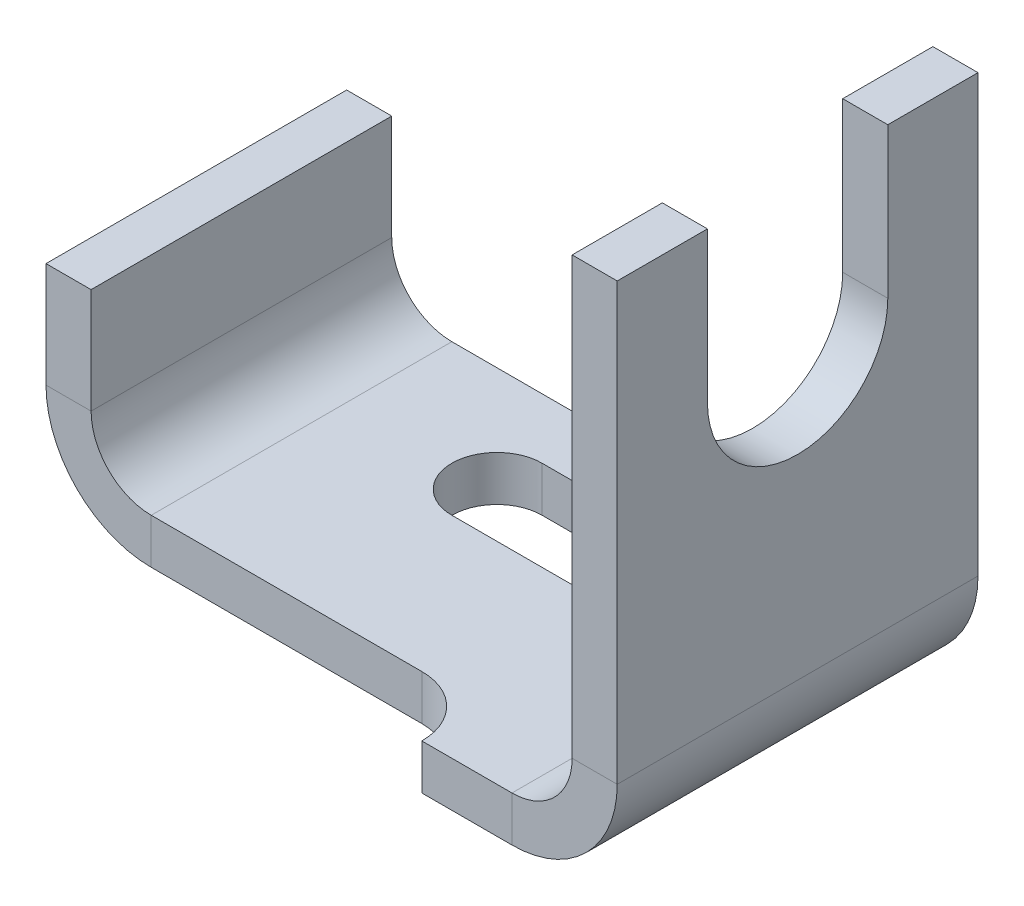
ISO-10303-21;
HEADER;
FILE_DESCRIPTION(('STEP AP214'),'2;1');
FILE_NAME('part.step','',(''),(''),'','','');
FILE_SCHEMA(('AUTOMOTIVE_DESIGN { 1 0 10303 214 1 1 1 1 }'));
ENDSEC;
DATA;
#1=APPLICATION_CONTEXT('core data for automotive mechanical design processes');
#2=APPLICATION_PROTOCOL_DEFINITION('international standard','automotive_design',2000,#1);
#3=PRODUCT_CONTEXT('',#1,'mechanical');
#4=PRODUCT('Part','Part','',(#3));
#5=PRODUCT_RELATED_PRODUCT_CATEGORY('part','',(#4));
#6=PRODUCT_DEFINITION_FORMATION('','',#4);
#7=PRODUCT_DEFINITION_CONTEXT('part definition',#1,'design');
#8=PRODUCT_DEFINITION('design','',#6,#7);
#9=PRODUCT_DEFINITION_SHAPE('','',#8);
#10=(LENGTH_UNIT() NAMED_UNIT(*) SI_UNIT(.MILLI.,.METRE.));
#11=(NAMED_UNIT(*) PLANE_ANGLE_UNIT() SI_UNIT($,.RADIAN.));
#12=(NAMED_UNIT(*) SI_UNIT($,.STERADIAN.) SOLID_ANGLE_UNIT());
#13=UNCERTAINTY_MEASURE_WITH_UNIT(LENGTH_MEASURE(1.E-05),#10,'distance_accuracy_value','');
#14=(GEOMETRIC_REPRESENTATION_CONTEXT(3) GLOBAL_UNCERTAINTY_ASSIGNED_CONTEXT((#13)) GLOBAL_UNIT_ASSIGNED_CONTEXT((#10,
#11,#12)) REPRESENTATION_CONTEXT('',''));
#15=CARTESIAN_POINT('',(0.,0.,0.));
#16=DIRECTION('',(0.,0.,1.));
#17=DIRECTION('',(1.,0.,0.));
#18=AXIS2_PLACEMENT_3D('',#15,#16,#17);
#19=CARTESIAN_POINT('',(18.,7.,12.));
#20=DIRECTION('',(0.,0.,1.));
#21=DIRECTION('',(1.,0.,0.));
#22=AXIS2_PLACEMENT_3D('',#19,#20,#21);
#23=PLANE('',#22);
#24=DIRECTION('',(1.,0.,0.));
#25=VECTOR('',#24,1.);
#26=CARTESIAN_POINT('',(0.,3.,12.));
#27=LINE('',#26,#25);
#28=CARTESIAN_POINT('',(14.,3.,12.));
#29=VERTEX_POINT('',#28);
#30=CARTESIAN_POINT('',(8.,3.,12.));
#31=VERTEX_POINT('',#30);
#32=EDGE_CURVE('E308',#29,#31,#27,.F.);
#33=ORIENTED_EDGE('',*,*,#32,.T.);
#34=DIRECTION('',(0.,1.,0.));
#35=VECTOR('',#34,1.);
#36=CARTESIAN_POINT('',(8.,3.,12.));
#37=LINE('',#36,#35);
#38=CARTESIAN_POINT('',(8.,0.,12.));
#39=VERTEX_POINT('',#38);
#40=EDGE_CURVE('E191',#31,#39,#37,.F.);
#41=ORIENTED_EDGE('',*,*,#40,.T.);
#42=DIRECTION('',(-1.,0.,0.));
#43=VECTOR('',#42,1.);
#44=CARTESIAN_POINT('',(0.,0.,12.));
#45=LINE('',#44,#43);
#46=CARTESIAN_POINT('',(14.,0.,12.));
#47=VERTEX_POINT('',#46);
#48=EDGE_CURVE('E287',#47,#39,#45,.T.);
#49=ORIENTED_EDGE('',*,*,#48,.F.);
#50=DIRECTION('',(0.,1.,0.));
#51=VECTOR('',#50,1.);
#52=CARTESIAN_POINT('',(14.,0.,12.));
#53=LINE('',#52,#51);
#54=EDGE_CURVE('E11',#47,#29,#53,.T.);
#55=ORIENTED_EDGE('',*,*,#54,.T.);
#56=EDGE_LOOP('',(#33,#41,#49,#55));
#57=FACE_BOUND('',#56,.T.);
#58=ADVANCED_FACE('F41',(#57),#23,.T.);
#59=CARTESIAN_POINT('',(-18.,0.,12.));
#60=DIRECTION('',(-1.,0.,0.));
#61=DIRECTION('',(0.,0.,1.));
#62=AXIS2_PLACEMENT_3D('',#59,#60,#61);
#63=PLANE('',#62);
#64=DIRECTION('',(0.,1.,0.));
#65=VECTOR('',#64,1.);
#66=CARTESIAN_POINT('',(-18.,0.,8.));
#67=LINE('',#66,#65);
#68=CARTESIAN_POINT('',(-18.,7.,8.));
#69=VERTEX_POINT('',#68);
#70=CARTESIAN_POINT('',(-18.,14.,8.));
#71=VERTEX_POINT('',#70);
#72=EDGE_CURVE('E227',#69,#71,#67,.T.);
#73=ORIENTED_EDGE('',*,*,#72,.F.);
#74=DIRECTION('',(0.,0.,-1.));
#75=VECTOR('',#74,1.);
#76=CARTESIAN_POINT('',(-18.,7.,12.));
#77=LINE('',#76,#75);
#78=CARTESIAN_POINT('',(-18.,7.,-12.));
#79=VERTEX_POINT('',#78);
#80=EDGE_CURVE('E309',#69,#79,#77,.T.);
#81=ORIENTED_EDGE('',*,*,#80,.T.);
#82=DIRECTION('',(0.,1.,0.));
#83=VECTOR('',#82,1.);
#84=CARTESIAN_POINT('',(-18.,0.,-12.));
#85=LINE('',#84,#83);
#86=CARTESIAN_POINT('',(-18.,14.,-12.));
#87=VERTEX_POINT('',#86);
#88=EDGE_CURVE('E282',#79,#87,#85,.T.);
#89=ORIENTED_EDGE('',*,*,#88,.T.);
#90=DIRECTION('',(0.,0.,-1.));
#91=VECTOR('',#90,1.);
#92=CARTESIAN_POINT('',(-18.,14.,12.));
#93=LINE('',#92,#91);
#94=EDGE_CURVE('E375',#71,#87,#93,.T.);
#95=ORIENTED_EDGE('',*,*,#94,.F.);
#96=EDGE_LOOP('',(#73,#81,#89,#95));
#97=FACE_BOUND('',#96,.T.);
#98=ADVANCED_FACE('F455',(#97),#63,.F.);
#99=CARTESIAN_POINT('',(-21.,14.,12.));
#100=DIRECTION('',(0.,1.,0.));
#101=DIRECTION('',(0.,0.,1.));
#102=AXIS2_PLACEMENT_3D('',#99,#100,#101);
#103=PLANE('',#102);
#104=DIRECTION('',(0.,0.,-1.));
#105=VECTOR('',#104,1.);
#106=CARTESIAN_POINT('',(-21.,14.,12.));
#107=LINE('',#106,#105);
#108=CARTESIAN_POINT('',(-21.,14.,8.));
#109=VERTEX_POINT('',#108);
#110=CARTESIAN_POINT('',(-21.,14.,-12.));
#111=VERTEX_POINT('',#110);
#112=EDGE_CURVE('E369',#109,#111,#107,.T.);
#113=ORIENTED_EDGE('',*,*,#112,.F.);
#114=DIRECTION('',(-1.,0.,0.));
#115=VECTOR('',#114,1.);
#116=CARTESIAN_POINT('',(-21.,14.,8.));
#117=LINE('',#116,#115);
#118=EDGE_CURVE('E230',#109,#71,#117,.F.);
#119=ORIENTED_EDGE('',*,*,#118,.T.);
#120=ORIENTED_EDGE('',*,*,#94,.T.);
#121=DIRECTION('',(1.,0.,0.));
#122=VECTOR('',#121,1.);
#123=CARTESIAN_POINT('',(-21.,14.,-12.));
#124=LINE('',#123,#122);
#125=EDGE_CURVE('E312',#111,#87,#124,.T.);
#126=ORIENTED_EDGE('',*,*,#125,.F.);
#127=EDGE_LOOP('',(#113,#119,#120,#126));
#128=FACE_BOUND('',#127,.T.);
#129=ADVANCED_FACE('F456',(#128),#103,.T.);
#130=CARTESIAN_POINT('',(-21.,0.,12.));
#131=DIRECTION('',(-1.,0.,0.));
#132=DIRECTION('',(0.,0.,1.));
#133=AXIS2_PLACEMENT_3D('',#130,#131,#132);
#134=PLANE('',#133);
#135=DIRECTION('',(0.,0.,-1.));
#136=VECTOR('',#135,1.);
#137=CARTESIAN_POINT('',(-21.,7.,12.));
#138=LINE('',#137,#136);
#139=CARTESIAN_POINT('',(-21.,7.00000000000001,8.));
#140=VERTEX_POINT('',#139);
#141=CARTESIAN_POINT('',(-21.,7.,-12.));
#142=VERTEX_POINT('',#141);
#143=EDGE_CURVE('E368',#140,#142,#138,.T.);
#144=ORIENTED_EDGE('',*,*,#143,.F.);
#145=DIRECTION('',(0.,1.,0.));
#146=VECTOR('',#145,1.);
#147=CARTESIAN_POINT('',(-21.,0.,8.));
#148=LINE('',#147,#146);
#149=EDGE_CURVE('E222',#140,#109,#148,.T.);
#150=ORIENTED_EDGE('',*,*,#149,.T.);
#151=ORIENTED_EDGE('',*,*,#112,.T.);
#152=DIRECTION('',(0.,1.,0.));
#153=VECTOR('',#152,1.);
#154=CARTESIAN_POINT('',(-21.,0.,-12.));
#155=LINE('',#154,#153);
#156=EDGE_CURVE('E317',#142,#111,#155,.T.);
#157=ORIENTED_EDGE('',*,*,#156,.F.);
#158=EDGE_LOOP('',(#144,#150,#151,#157));
#159=FACE_BOUND('',#158,.T.);
#160=ADVANCED_FACE('F476',(#159),#134,.T.);
#161=CARTESIAN_POINT('',(-14.,7.,12.));
#162=DIRECTION('',(0.,0.,-1.));
#163=DIRECTION('',(-1.,0.,0.));
#164=AXIS2_PLACEMENT_3D('',#161,#162,#163);
#165=CYLINDRICAL_SURFACE('',#164,7.);
#166=DIRECTION('',(0.,0.,-1.));
#167=VECTOR('',#166,1.);
#168=CARTESIAN_POINT('',(-14.,0.,12.));
#169=LINE('',#168,#167);
#170=CARTESIAN_POINT('',(-14.,0.,8.));
#171=VERTEX_POINT('',#170);
#172=CARTESIAN_POINT('',(-14.,0.,-12.));
#173=VERTEX_POINT('',#172);
#174=EDGE_CURVE('E366',#171,#173,#169,.T.);
#175=ORIENTED_EDGE('',*,*,#174,.F.);
#176=CARTESIAN_POINT('',(-14.,7.,8.));
#177=DIRECTION('',(0.,0.,-1.));
#178=DIRECTION('',(-1.,0.,0.));
#179=AXIS2_PLACEMENT_3D('',#176,#177,#178);
#180=CIRCLE('',#179,7.);
#181=EDGE_CURVE('E223',#171,#140,#180,.T.);
#182=ORIENTED_EDGE('',*,*,#181,.T.);
#183=ORIENTED_EDGE('',*,*,#143,.T.);
#184=CARTESIAN_POINT('',(-14.,7.,-12.));
#185=DIRECTION('',(0.,0.,1.));
#186=DIRECTION('',(1.,0.,0.));
#187=AXIS2_PLACEMENT_3D('',#184,#185,#186);
#188=CIRCLE('',#187,7.);
#189=EDGE_CURVE('E316',#173,#142,#188,.F.);
#190=ORIENTED_EDGE('',*,*,#189,.F.);
#191=EDGE_LOOP('',(#175,#182,#183,#190));
#192=FACE_BOUND('',#191,.T.);
#193=ADVANCED_FACE('F480',(#192),#165,.T.);
#194=CARTESIAN_POINT('',(0.,0.,12.));
#195=DIRECTION('',(0.,-1.,0.));
#196=DIRECTION('',(0.,0.,-1.));
#197=AXIS2_PLACEMENT_3D('',#194,#195,#196);
#198=PLANE('',#197);
#199=CARTESIAN_POINT('',(-3.99999999999999,0.,-5.));
#200=DIRECTION('',(0.,1.,0.));
#201=DIRECTION('',(-1.,0.,0.));
#202=AXIS2_PLACEMENT_3D('',#199,#200,#201);
#203=CIRCLE('',#202,3.);
#204=CARTESIAN_POINT('',(-3.99999999999999,0.,-8.));
#205=VERTEX_POINT('',#204);
#206=CARTESIAN_POINT('',(-3.99999999999999,0.,-2.));
#207=VERTEX_POINT('',#206);
#208=EDGE_CURVE('E231',#205,#207,#203,.T.);
#209=ORIENTED_EDGE('',*,*,#208,.T.);
#210=DIRECTION('',(1.,0.,0.));
#211=VECTOR('',#210,1.);
#212=CARTESIAN_POINT('',(-3.99999999999999,0.,-2.));
#213=LINE('',#212,#211);
#214=CARTESIAN_POINT('',(8.00000000000001,0.,-2.));
#215=VERTEX_POINT('',#214);
#216=EDGE_CURVE('E236',#207,#215,#213,.T.);
#217=ORIENTED_EDGE('',*,*,#216,.T.);
#218=CARTESIAN_POINT('',(8.00000000000001,0.,-5.));
#219=DIRECTION('',(0.,1.,0.));
#220=DIRECTION('',(-1.,0.,0.));
#221=AXIS2_PLACEMENT_3D('',#218,#219,#220);
#222=CIRCLE('',#221,3.);
#223=CARTESIAN_POINT('',(8.00000000000001,0.,-8.));
#224=VERTEX_POINT('',#223);
#225=EDGE_CURVE('E65',#215,#224,#222,.T.);
#226=ORIENTED_EDGE('',*,*,#225,.T.);
#227=DIRECTION('',(-1.,0.,0.));
#228=VECTOR('',#227,1.);
#229=CARTESIAN_POINT('',(-3.99999999999999,0.,-8.));
#230=LINE('',#229,#228);
#231=EDGE_CURVE('E241',#224,#205,#230,.T.);
#232=ORIENTED_EDGE('',*,*,#231,.T.);
#233=EDGE_LOOP('',(#209,#217,#226,#232));
#234=FACE_BOUND('',#233,.T.);
#235=ORIENTED_EDGE('',*,*,#48,.T.);
#236=CARTESIAN_POINT('',(4.,0.,12.));
#237=DIRECTION('',(0.,-1.,0.));
#238=DIRECTION('',(1.,0.,0.));
#239=AXIS2_PLACEMENT_3D('',#236,#237,#238);
#240=CIRCLE('',#239,4.);
#241=CARTESIAN_POINT('',(4.,0.,8.));
#242=VERTEX_POINT('',#241);
#243=EDGE_CURVE('E202',#242,#39,#240,.T.);
#244=ORIENTED_EDGE('',*,*,#243,.F.);
#245=DIRECTION('',(1.,0.,0.));
#246=VECTOR('',#245,1.);
#247=CARTESIAN_POINT('',(0.,0.,8.));
#248=LINE('',#247,#246);
#249=EDGE_CURVE('E204',#171,#242,#248,.T.);
#250=ORIENTED_EDGE('',*,*,#249,.F.);
#251=ORIENTED_EDGE('',*,*,#174,.T.);
#252=DIRECTION('',(-1.,0.,0.));
#253=VECTOR('',#252,1.);
#254=CARTESIAN_POINT('',(0.,0.,-12.));
#255=LINE('',#254,#253);
#256=CARTESIAN_POINT('',(14.,0.,-12.));
#257=VERTEX_POINT('',#256);
#258=EDGE_CURVE('E324',#257,#173,#255,.T.);
#259=ORIENTED_EDGE('',*,*,#258,.F.);
#260=DIRECTION('',(0.,0.,-1.));
#261=VECTOR('',#260,1.);
#262=CARTESIAN_POINT('',(14.,0.,12.));
#263=LINE('',#262,#261);
#264=EDGE_CURVE('E361',#47,#257,#263,.T.);
#265=ORIENTED_EDGE('',*,*,#264,.F.);
#266=EDGE_LOOP('',(#235,#244,#250,#251,#259,#265));
#267=FACE_BOUND('',#266,.T.);
#268=ADVANCED_FACE('F415',(#234,#267),#198,.T.);
#269=CARTESIAN_POINT('',(0.,3.,12.));
#270=DIRECTION('',(0.,-1.,0.));
#271=DIRECTION('',(1.,0.,0.));
#272=AXIS2_PLACEMENT_3D('',#269,#270,#271);
#273=PLANE('',#272);
#274=DIRECTION('',(1.,0.,0.));
#275=VECTOR('',#274,1.);
#276=CARTESIAN_POINT('',(-3.99999999999999,3.,-2.));
#277=LINE('',#276,#275);
#278=CARTESIAN_POINT('',(-3.99999999999999,3.,-2.));
#279=VERTEX_POINT('',#278);
#280=CARTESIAN_POINT('',(8.00000000000001,3.,-2.));
#281=VERTEX_POINT('',#280);
#282=EDGE_CURVE('E246',#279,#281,#277,.T.);
#283=ORIENTED_EDGE('',*,*,#282,.F.);
#284=CARTESIAN_POINT('',(-3.99999999999999,3.,-5.));
#285=DIRECTION('',(0.,1.,0.));
#286=DIRECTION('',(-1.,0.,0.));
#287=AXIS2_PLACEMENT_3D('',#284,#285,#286);
#288=CIRCLE('',#287,3.);
#289=CARTESIAN_POINT('',(-3.99999999999999,3.,-8.));
#290=VERTEX_POINT('',#289);
#291=EDGE_CURVE('E235',#290,#279,#288,.T.);
#292=ORIENTED_EDGE('',*,*,#291,.F.);
#293=DIRECTION('',(-1.,0.,0.));
#294=VECTOR('',#293,1.);
#295=CARTESIAN_POINT('',(-3.99999999999999,3.,-8.));
#296=LINE('',#295,#294);
#297=CARTESIAN_POINT('',(8.00000000000001,3.,-8.));
#298=VERTEX_POINT('',#297);
#299=EDGE_CURVE('E240',#298,#290,#296,.T.);
#300=ORIENTED_EDGE('',*,*,#299,.F.);
#301=CARTESIAN_POINT('',(8.00000000000001,3.,-5.));
#302=DIRECTION('',(0.,1.,0.));
#303=DIRECTION('',(-1.,0.,0.));
#304=AXIS2_PLACEMENT_3D('',#301,#302,#303);
#305=CIRCLE('',#304,3.);
#306=EDGE_CURVE('E248',#281,#298,#305,.T.);
#307=ORIENTED_EDGE('',*,*,#306,.F.);
#308=EDGE_LOOP('',(#283,#292,#300,#307));
#309=FACE_BOUND('',#308,.T.);
#310=CARTESIAN_POINT('',(4.,3.,12.));
#311=DIRECTION('',(0.,-1.,0.));
#312=DIRECTION('',(1.,0.,0.));
#313=AXIS2_PLACEMENT_3D('',#310,#311,#312);
#314=CIRCLE('',#313,4.);
#315=CARTESIAN_POINT('',(4.,3.,8.));
#316=VERTEX_POINT('',#315);
#317=EDGE_CURVE('E188',#316,#31,#314,.T.);
#318=ORIENTED_EDGE('',*,*,#317,.T.);
#319=ORIENTED_EDGE('',*,*,#32,.F.);
#320=DIRECTION('',(0.,0.,-1.));
#321=VECTOR('',#320,1.);
#322=CARTESIAN_POINT('',(14.,3.,12.));
#323=LINE('',#322,#321);
#324=CARTESIAN_POINT('',(14.,3.,-12.));
#325=VERTEX_POINT('',#324);
#326=EDGE_CURVE('E346',#29,#325,#323,.T.);
#327=ORIENTED_EDGE('',*,*,#326,.T.);
#328=DIRECTION('',(-1.,0.,0.));
#329=VECTOR('',#328,1.);
#330=CARTESIAN_POINT('',(0.,3.,-12.));
#331=LINE('',#330,#329);
#332=CARTESIAN_POINT('',(-14.,3.,-12.));
#333=VERTEX_POINT('',#332);
#334=EDGE_CURVE('E338',#325,#333,#331,.T.);
#335=ORIENTED_EDGE('',*,*,#334,.T.);
#336=DIRECTION('',(0.,0.,-1.));
#337=VECTOR('',#336,1.);
#338=CARTESIAN_POINT('',(-14.,3.,12.));
#339=LINE('',#338,#337);
#340=CARTESIAN_POINT('',(-14.,3.,8.));
#341=VERTEX_POINT('',#340);
#342=EDGE_CURVE('E206',#341,#333,#339,.T.);
#343=ORIENTED_EDGE('',*,*,#342,.F.);
#344=DIRECTION('',(1.,0.,0.));
#345=VECTOR('',#344,1.);
#346=CARTESIAN_POINT('',(0.,3.,8.));
#347=LINE('',#346,#345);
#348=EDGE_CURVE('E57',#341,#316,#347,.T.);
#349=ORIENTED_EDGE('',*,*,#348,.T.);
#350=EDGE_LOOP('',(#318,#319,#327,#335,#343,#349));
#351=FACE_BOUND('',#350,.T.);
#352=ADVANCED_FACE('F207',(#309,#351),#273,.F.);
#353=CARTESIAN_POINT('',(-14.,7.,12.));
#354=DIRECTION('',(0.,0.,-1.));
#355=DIRECTION('',(-1.,0.,0.));
#356=AXIS2_PLACEMENT_3D('',#353,#354,#355);
#357=CYLINDRICAL_SURFACE('',#356,4.);
#358=CARTESIAN_POINT('',(-14.,7.,8.));
#359=DIRECTION('',(0.,0.,-1.));
#360=DIRECTION('',(-1.,0.,0.));
#361=AXIS2_PLACEMENT_3D('',#358,#359,#360);
#362=CIRCLE('',#361,4.);
#363=EDGE_CURVE('E216',#341,#69,#362,.T.);
#364=ORIENTED_EDGE('',*,*,#363,.F.);
#365=ORIENTED_EDGE('',*,*,#342,.T.);
#366=CARTESIAN_POINT('',(-14.,7.,-12.));
#367=DIRECTION('',(0.,0.,1.));
#368=DIRECTION('',(1.,0.,0.));
#369=AXIS2_PLACEMENT_3D('',#366,#367,#368);
#370=CIRCLE('',#369,4.);
#371=EDGE_CURVE('E291',#333,#79,#370,.F.);
#372=ORIENTED_EDGE('',*,*,#371,.T.);
#373=ORIENTED_EDGE('',*,*,#80,.F.);
#374=EDGE_LOOP('',(#364,#365,#372,#373));
#375=FACE_BOUND('',#374,.T.);
#376=ADVANCED_FACE('F497',(#375),#357,.F.);
#377=CARTESIAN_POINT('',(18.,36.,12.));
#378=DIRECTION('',(0.,1.,0.));
#379=DIRECTION('',(0.,0.,1.));
#380=AXIS2_PLACEMENT_3D('',#377,#378,#379);
#381=PLANE('',#380);
#382=DIRECTION('',(-1.,0.,0.));
#383=VECTOR('',#382,1.);
#384=CARTESIAN_POINT('',(21.,36.,6.));
#385=LINE('',#384,#383);
#386=CARTESIAN_POINT('',(21.,36.,6.));
#387=VERTEX_POINT('',#386);
#388=CARTESIAN_POINT('',(18.,36.,6.));
#389=VERTEX_POINT('',#388);
#390=EDGE_CURVE('E271',#387,#389,#385,.T.);
#391=ORIENTED_EDGE('',*,*,#390,.T.);
#392=DIRECTION('',(0.,0.,-1.));
#393=VECTOR('',#392,1.);
#394=CARTESIAN_POINT('',(18.,36.,12.));
#395=LINE('',#394,#393);
#396=CARTESIAN_POINT('',(18.,36.,12.));
#397=VERTEX_POINT('',#396);
#398=EDGE_CURVE('E351',#397,#389,#395,.T.);
#399=ORIENTED_EDGE('',*,*,#398,.F.);
#400=DIRECTION('',(1.,0.,0.));
#401=VECTOR('',#400,1.);
#402=CARTESIAN_POINT('',(18.,36.,12.));
#403=LINE('',#402,#401);
#404=CARTESIAN_POINT('',(21.,36.,12.));
#405=VERTEX_POINT('',#404);
#406=EDGE_CURVE('E299',#397,#405,#403,.T.);
#407=ORIENTED_EDGE('',*,*,#406,.T.);
#408=DIRECTION('',(0.,0.,-1.));
#409=VECTOR('',#408,1.);
#410=CARTESIAN_POINT('',(21.,36.,12.));
#411=LINE('',#410,#409);
#412=EDGE_CURVE('E357',#405,#387,#411,.T.);
#413=ORIENTED_EDGE('',*,*,#412,.T.);
#414=EDGE_LOOP('',(#391,#399,#407,#413));
#415=FACE_BOUND('',#414,.T.);
#416=ADVANCED_FACE('F402',(#415),#381,.T.);
#417=CARTESIAN_POINT('',(14.,0.,12.));
#418=DIRECTION('',(0.,0.,1.));
#419=DIRECTION('',(1.,0.,0.));
#420=AXIS2_PLACEMENT_3D('',#417,#418,#419);
#421=PLANE('',#420);
#422=ORIENTED_EDGE('',*,*,#54,.F.);
#423=CARTESIAN_POINT('',(14.,7.,12.));
#424=DIRECTION('',(0.,0.,1.));
#425=DIRECTION('',(1.,0.,0.));
#426=AXIS2_PLACEMENT_3D('',#423,#424,#425);
#427=CIRCLE('',#426,7.);
#428=CARTESIAN_POINT('',(21.,7.,12.));
#429=VERTEX_POINT('',#428);
#430=EDGE_CURVE('E292',#429,#47,#427,.F.);
#431=ORIENTED_EDGE('',*,*,#430,.F.);
#432=DIRECTION('',(1.,0.,0.));
#433=VECTOR('',#432,1.);
#434=CARTESIAN_POINT('',(18.,7.,12.));
#435=LINE('',#434,#433);
#436=CARTESIAN_POINT('',(18.,7.,12.));
#437=VERTEX_POINT('',#436);
#438=EDGE_CURVE('E47',#437,#429,#435,.T.);
#439=ORIENTED_EDGE('',*,*,#438,.F.);
#440=CARTESIAN_POINT('',(14.,7.,12.));
#441=DIRECTION('',(0.,0.,1.));
#442=DIRECTION('',(1.,0.,0.));
#443=AXIS2_PLACEMENT_3D('',#440,#441,#442);
#444=CIRCLE('',#443,4.);
#445=EDGE_CURVE('E304',#437,#29,#444,.F.);
#446=ORIENTED_EDGE('',*,*,#445,.T.);
#447=EDGE_LOOP('',(#422,#431,#439,#446));
#448=FACE_BOUND('',#447,.T.);
#449=ADVANCED_FACE('F43',(#448),#421,.T.);
#450=CARTESIAN_POINT('',(21.,7.,-12.));
#451=DIRECTION('',(0.,0.,-1.));
#452=DIRECTION('',(-1.,0.,0.));
#453=AXIS2_PLACEMENT_3D('',#450,#451,#452);
#454=PLANE('',#453);
#455=DIRECTION('',(-1.,0.,0.));
#456=VECTOR('',#455,1.);
#457=CARTESIAN_POINT('',(21.,7.,-12.));
#458=LINE('',#457,#456);
#459=CARTESIAN_POINT('',(21.,7.,-12.));
#460=VERTEX_POINT('',#459);
#461=CARTESIAN_POINT('',(18.,7.,-12.));
#462=VERTEX_POINT('',#461);
#463=EDGE_CURVE('E385',#460,#462,#458,.T.);
#464=ORIENTED_EDGE('',*,*,#463,.F.);
#465=CARTESIAN_POINT('',(14.,7.,-12.));
#466=DIRECTION('',(0.,0.,1.));
#467=DIRECTION('',(1.,0.,0.));
#468=AXIS2_PLACEMENT_3D('',#465,#466,#467);
#469=CIRCLE('',#468,7.);
#470=EDGE_CURVE('E321',#460,#257,#469,.F.);
#471=ORIENTED_EDGE('',*,*,#470,.T.);
#472=DIRECTION('',(0.,-1.,0.));
#473=VECTOR('',#472,1.);
#474=CARTESIAN_POINT('',(14.,3.,-12.));
#475=LINE('',#474,#473);
#476=EDGE_CURVE('E379',#325,#257,#475,.T.);
#477=ORIENTED_EDGE('',*,*,#476,.F.);
#478=CARTESIAN_POINT('',(14.,7.,-12.));
#479=DIRECTION('',(0.,0.,1.));
#480=DIRECTION('',(1.,0.,0.));
#481=AXIS2_PLACEMENT_3D('',#478,#479,#480);
#482=CIRCLE('',#481,4.);
#483=EDGE_CURVE('E340',#462,#325,#482,.F.);
#484=ORIENTED_EDGE('',*,*,#483,.F.);
#485=EDGE_LOOP('',(#464,#471,#477,#484));
#486=FACE_BOUND('',#485,.T.);
#487=ADVANCED_FACE('F423',(#486),#454,.T.);
#488=CARTESIAN_POINT('',(14.,3.,-12.));
#489=DIRECTION('',(0.,0.,-1.));
#490=DIRECTION('',(-1.,0.,0.));
#491=AXIS2_PLACEMENT_3D('',#488,#489,#490);
#492=PLANE('',#491);
#493=DIRECTION('',(0.,-1.,0.));
#494=VECTOR('',#493,1.);
#495=CARTESIAN_POINT('',(21.,0.,-12.));
#496=LINE('',#495,#494);
#497=CARTESIAN_POINT('',(21.,36.,-12.));
#498=VERTEX_POINT('',#497);
#499=EDGE_CURVE('E330',#498,#460,#496,.T.);
#500=ORIENTED_EDGE('',*,*,#499,.T.);
#501=ORIENTED_EDGE('',*,*,#463,.T.);
#502=DIRECTION('',(0.,1.,0.));
#503=VECTOR('',#502,1.);
#504=CARTESIAN_POINT('',(18.,0.,-12.));
#505=LINE('',#504,#503);
#506=CARTESIAN_POINT('',(18.,36.,-12.));
#507=VERTEX_POINT('',#506);
#508=EDGE_CURVE('E335',#507,#462,#505,.F.);
#509=ORIENTED_EDGE('',*,*,#508,.F.);
#510=DIRECTION('',(1.,0.,0.));
#511=VECTOR('',#510,1.);
#512=CARTESIAN_POINT('',(18.,36.,-12.));
#513=LINE('',#512,#511);
#514=EDGE_CURVE('E333',#507,#498,#513,.T.);
#515=ORIENTED_EDGE('',*,*,#514,.T.);
#516=EDGE_LOOP('',(#500,#501,#509,#515));
#517=FACE_BOUND('',#516,.T.);
#518=ADVANCED_FACE('F425',(#517),#492,.T.);
#519=CARTESIAN_POINT('',(-14.,0.,-12.));
#520=DIRECTION('',(0.,0.,-1.));
#521=DIRECTION('',(-1.,0.,0.));
#522=AXIS2_PLACEMENT_3D('',#519,#520,#521);
#523=PLANE('',#522);
#524=DIRECTION('',(0.,1.,0.));
#525=VECTOR('',#524,1.);
#526=CARTESIAN_POINT('',(-14.,0.,-12.));
#527=LINE('',#526,#525);
#528=EDGE_CURVE('E380',#173,#333,#527,.T.);
#529=ORIENTED_EDGE('',*,*,#528,.F.);
#530=ORIENTED_EDGE('',*,*,#189,.T.);
#531=DIRECTION('',(-1.,0.,0.));
#532=VECTOR('',#531,1.);
#533=CARTESIAN_POINT('',(-18.,7.,-12.));
#534=LINE('',#533,#532);
#535=EDGE_CURVE('E372',#79,#142,#534,.T.);
#536=ORIENTED_EDGE('',*,*,#535,.F.);
#537=ORIENTED_EDGE('',*,*,#371,.F.);
#538=EDGE_LOOP('',(#529,#530,#536,#537));
#539=FACE_BOUND('',#538,.T.);
#540=ADVANCED_FACE('F470',(#539),#523,.T.);
#541=CARTESIAN_POINT('',(-18.,7.,-12.));
#542=DIRECTION('',(0.,0.,-1.));
#543=DIRECTION('',(-1.,0.,0.));
#544=AXIS2_PLACEMENT_3D('',#541,#542,#543);
#545=PLANE('',#544);
#546=ORIENTED_EDGE('',*,*,#258,.T.);
#547=ORIENTED_EDGE('',*,*,#528,.T.);
#548=ORIENTED_EDGE('',*,*,#334,.F.);
#549=ORIENTED_EDGE('',*,*,#476,.T.);
#550=EDGE_LOOP('',(#546,#547,#548,#549));
#551=FACE_BOUND('',#550,.T.);
#552=ADVANCED_FACE('F468',(#551),#545,.T.);
#553=CARTESIAN_POINT('',(14.,7.,12.));
#554=DIRECTION('',(0.,0.,-1.));
#555=DIRECTION('',(-1.,0.,0.));
#556=AXIS2_PLACEMENT_3D('',#553,#554,#555);
#557=CYLINDRICAL_SURFACE('',#556,7.);
#558=ORIENTED_EDGE('',*,*,#470,.F.);
#559=DIRECTION('',(0.,0.,-1.));
#560=VECTOR('',#559,1.);
#561=CARTESIAN_POINT('',(21.,7.,12.));
#562=LINE('',#561,#560);
#563=EDGE_CURVE('E359',#429,#460,#562,.T.);
#564=ORIENTED_EDGE('',*,*,#563,.F.);
#565=ORIENTED_EDGE('',*,*,#430,.T.);
#566=ORIENTED_EDGE('',*,*,#264,.T.);
#567=EDGE_LOOP('',(#558,#564,#565,#566));
#568=FACE_BOUND('',#567,.T.);
#569=ADVANCED_FACE('F391',(#568),#557,.T.);
#570=CARTESIAN_POINT('',(21.,0.,12.));
#571=DIRECTION('',(1.,0.,0.));
#572=DIRECTION('',(0.,0.,-1.));
#573=AXIS2_PLACEMENT_3D('',#570,#571,#572);
#574=PLANE('',#573);
#575=DIRECTION('',(0.,1.,0.));
#576=VECTOR('',#575,1.);
#577=CARTESIAN_POINT('',(21.,36.,6.));
#578=LINE('',#577,#576);
#579=CARTESIAN_POINT('',(21.,26.,6.));
#580=VERTEX_POINT('',#579);
#581=EDGE_CURVE('E265',#580,#387,#578,.T.);
#582=ORIENTED_EDGE('',*,*,#581,.T.);
#583=ORIENTED_EDGE('',*,*,#412,.F.);
#584=DIRECTION('',(0.,-1.,0.));
#585=VECTOR('',#584,1.);
#586=CARTESIAN_POINT('',(21.,0.,12.));
#587=LINE('',#586,#585);
#588=EDGE_CURVE('E298',#405,#429,#587,.T.);
#589=ORIENTED_EDGE('',*,*,#588,.T.);
#590=ORIENTED_EDGE('',*,*,#563,.T.);
#591=ORIENTED_EDGE('',*,*,#499,.F.);
#592=CARTESIAN_POINT('',(21.,36.,-6.));
#593=VERTEX_POINT('',#592);
#594=EDGE_CURVE('E358',#593,#498,#411,.T.);
#595=ORIENTED_EDGE('',*,*,#594,.F.);
#596=DIRECTION('',(0.,-1.,0.));
#597=VECTOR('',#596,1.);
#598=CARTESIAN_POINT('',(21.,26.,-6.));
#599=LINE('',#598,#597);
#600=CARTESIAN_POINT('',(21.,26.,-6.));
#601=VERTEX_POINT('',#600);
#602=EDGE_CURVE('E268',#593,#601,#599,.T.);
#603=ORIENTED_EDGE('',*,*,#602,.T.);
#604=CARTESIAN_POINT('',(21.,26.,0.));
#605=DIRECTION('',(-1.,0.,0.));
#606=DIRECTION('',(0.,0.,1.));
#607=AXIS2_PLACEMENT_3D('',#604,#605,#606);
#608=CIRCLE('',#607,6.);
#609=EDGE_CURVE('E266',#601,#580,#608,.T.);
#610=ORIENTED_EDGE('',*,*,#609,.T.);
#611=EDGE_LOOP('',(#582,#583,#589,#590,#591,#595,#603,#610));
#612=FACE_BOUND('',#611,.T.);
#613=ADVANCED_FACE('F397',(#612),#574,.T.);
#614=DIRECTION('',(-1.,0.,0.));
#615=VECTOR('',#614,1.);
#616=CARTESIAN_POINT('',(21.,36.,-6.));
#617=LINE('',#616,#615);
#618=CARTESIAN_POINT('',(18.,36.,-6.));
#619=VERTEX_POINT('',#618);
#620=EDGE_CURVE('E285',#593,#619,#617,.T.);
#621=ORIENTED_EDGE('',*,*,#620,.F.);
#622=ORIENTED_EDGE('',*,*,#594,.T.);
#623=ORIENTED_EDGE('',*,*,#514,.F.);
#624=EDGE_CURVE('E355',#619,#507,#395,.T.);
#625=ORIENTED_EDGE('',*,*,#624,.F.);
#626=EDGE_LOOP('',(#621,#622,#623,#625));
#627=FACE_BOUND('',#626,.T.);
#628=ADVANCED_FACE('F429',(#627),#381,.T.);
#629=CARTESIAN_POINT('',(18.,0.,12.));
#630=DIRECTION('',(1.,0.,0.));
#631=DIRECTION('',(0.,0.,-1.));
#632=AXIS2_PLACEMENT_3D('',#629,#630,#631);
#633=PLANE('',#632);
#634=ORIENTED_EDGE('',*,*,#398,.T.);
#635=DIRECTION('',(0.,1.,0.));
#636=VECTOR('',#635,1.);
#637=CARTESIAN_POINT('',(18.,36.,6.));
#638=LINE('',#637,#636);
#639=CARTESIAN_POINT('',(18.,26.,6.));
#640=VERTEX_POINT('',#639);
#641=EDGE_CURVE('E258',#640,#389,#638,.T.);
#642=ORIENTED_EDGE('',*,*,#641,.F.);
#643=CARTESIAN_POINT('',(18.,26.,0.));
#644=DIRECTION('',(-1.,0.,0.));
#645=DIRECTION('',(0.,0.,1.));
#646=AXIS2_PLACEMENT_3D('',#643,#644,#645);
#647=CIRCLE('',#646,6.);
#648=CARTESIAN_POINT('',(18.,26.,-6.));
#649=VERTEX_POINT('',#648);
#650=EDGE_CURVE('E269',#649,#640,#647,.T.);
#651=ORIENTED_EDGE('',*,*,#650,.F.);
#652=DIRECTION('',(0.,-1.,0.));
#653=VECTOR('',#652,1.);
#654=CARTESIAN_POINT('',(18.,26.,-6.));
#655=LINE('',#654,#653);
#656=EDGE_CURVE('E273',#619,#649,#655,.T.);
#657=ORIENTED_EDGE('',*,*,#656,.F.);
#658=ORIENTED_EDGE('',*,*,#624,.T.);
#659=ORIENTED_EDGE('',*,*,#508,.T.);
#660=DIRECTION('',(0.,0.,-1.));
#661=VECTOR('',#660,1.);
#662=CARTESIAN_POINT('',(18.,7.,12.));
#663=LINE('',#662,#661);
#664=EDGE_CURVE('E348',#437,#462,#663,.T.);
#665=ORIENTED_EDGE('',*,*,#664,.F.);
#666=DIRECTION('',(0.,1.,0.));
#667=VECTOR('',#666,1.);
#668=CARTESIAN_POINT('',(18.,0.,12.));
#669=LINE('',#668,#667);
#670=EDGE_CURVE('E305',#397,#437,#669,.F.);
#671=ORIENTED_EDGE('',*,*,#670,.F.);
#672=EDGE_LOOP('',(#634,#642,#651,#657,#658,#659,#665,#671));
#673=FACE_BOUND('',#672,.T.);
#674=ADVANCED_FACE('F404',(#673),#633,.F.);
#675=CARTESIAN_POINT('',(14.,7.,12.));
#676=DIRECTION('',(0.,0.,-1.));
#677=DIRECTION('',(-1.,0.,0.));
#678=AXIS2_PLACEMENT_3D('',#675,#676,#677);
#679=CYLINDRICAL_SURFACE('',#678,4.);
#680=ORIENTED_EDGE('',*,*,#483,.T.);
#681=ORIENTED_EDGE('',*,*,#326,.F.);
#682=ORIENTED_EDGE('',*,*,#445,.F.);
#683=ORIENTED_EDGE('',*,*,#664,.T.);
#684=EDGE_LOOP('',(#680,#681,#682,#683));
#685=FACE_BOUND('',#684,.T.);
#686=ADVANCED_FACE('F406',(#685),#679,.F.);
#687=CARTESIAN_POINT('',(-14.,7.,12.));
#688=DIRECTION('',(0.,0.,1.));
#689=DIRECTION('',(1.,0.,0.));
#690=AXIS2_PLACEMENT_3D('',#687,#688,#689);
#691=PLANE('',#690);
#692=ORIENTED_EDGE('',*,*,#670,.T.);
#693=ORIENTED_EDGE('',*,*,#438,.T.);
#694=ORIENTED_EDGE('',*,*,#588,.F.);
#695=ORIENTED_EDGE('',*,*,#406,.F.);
#696=EDGE_LOOP('',(#692,#693,#694,#695));
#697=FACE_BOUND('',#696,.T.);
#698=ADVANCED_FACE('F388',(#697),#691,.T.);
#699=CARTESIAN_POINT('',(-14.,7.,-12.));
#700=DIRECTION('',(0.,0.,1.));
#701=DIRECTION('',(1.,0.,0.));
#702=AXIS2_PLACEMENT_3D('',#699,#700,#701);
#703=PLANE('',#702);
#704=ORIENTED_EDGE('',*,*,#88,.F.);
#705=ORIENTED_EDGE('',*,*,#535,.T.);
#706=ORIENTED_EDGE('',*,*,#156,.T.);
#707=ORIENTED_EDGE('',*,*,#125,.T.);
#708=EDGE_LOOP('',(#704,#705,#706,#707));
#709=FACE_BOUND('',#708,.T.);
#710=ADVANCED_FACE('F441',(#709),#703,.F.);
#711=CARTESIAN_POINT('',(21.,36.,6.));
#712=DIRECTION('',(0.,0.,1.));
#713=DIRECTION('',(0.,-1.,0.));
#714=AXIS2_PLACEMENT_3D('',#711,#712,#713);
#715=PLANE('',#714);
#716=ORIENTED_EDGE('',*,*,#641,.T.);
#717=ORIENTED_EDGE('',*,*,#390,.F.);
#718=ORIENTED_EDGE('',*,*,#581,.F.);
#719=DIRECTION('',(-1.,0.,0.));
#720=VECTOR('',#719,1.);
#721=CARTESIAN_POINT('',(21.,26.,6.));
#722=LINE('',#721,#720);
#723=EDGE_CURVE('E276',#580,#640,#722,.T.);
#724=ORIENTED_EDGE('',*,*,#723,.T.);
#725=EDGE_LOOP('',(#716,#717,#718,#724));
#726=FACE_BOUND('',#725,.T.);
#727=ADVANCED_FACE('F437',(#726),#715,.F.);
#728=CARTESIAN_POINT('',(21.,26.,0.));
#729=DIRECTION('',(-1.,0.,0.));
#730=DIRECTION('',(0.,0.,1.));
#731=AXIS2_PLACEMENT_3D('',#728,#729,#730);
#732=CYLINDRICAL_SURFACE('',#731,6.);
#733=ORIENTED_EDGE('',*,*,#650,.T.);
#734=ORIENTED_EDGE('',*,*,#723,.F.);
#735=ORIENTED_EDGE('',*,*,#609,.F.);
#736=DIRECTION('',(-1.,0.,0.));
#737=VECTOR('',#736,1.);
#738=CARTESIAN_POINT('',(21.,26.,-6.));
#739=LINE('',#738,#737);
#740=EDGE_CURVE('E284',#601,#649,#739,.T.);
#741=ORIENTED_EDGE('',*,*,#740,.T.);
#742=EDGE_LOOP('',(#733,#734,#735,#741));
#743=FACE_BOUND('',#742,.T.);
#744=ADVANCED_FACE('F436',(#743),#732,.F.);
#745=CARTESIAN_POINT('',(21.,26.,-6.));
#746=DIRECTION('',(0.,0.,-1.));
#747=DIRECTION('',(0.,1.,0.));
#748=AXIS2_PLACEMENT_3D('',#745,#746,#747);
#749=PLANE('',#748);
#750=ORIENTED_EDGE('',*,*,#656,.T.);
#751=ORIENTED_EDGE('',*,*,#740,.F.);
#752=ORIENTED_EDGE('',*,*,#602,.F.);
#753=ORIENTED_EDGE('',*,*,#620,.T.);
#754=EDGE_LOOP('',(#750,#751,#752,#753));
#755=FACE_BOUND('',#754,.T.);
#756=ADVANCED_FACE('F433',(#755),#749,.F.);
#757=CARTESIAN_POINT('',(-3.99999999999999,0.,-5.));
#758=DIRECTION('',(0.,1.,0.));
#759=DIRECTION('',(-1.,0.,0.));
#760=AXIS2_PLACEMENT_3D('',#757,#758,#759);
#761=CYLINDRICAL_SURFACE('',#760,3.);
#762=ORIENTED_EDGE('',*,*,#291,.T.);
#763=DIRECTION('',(0.,1.,0.));
#764=VECTOR('',#763,1.);
#765=CARTESIAN_POINT('',(-3.99999999999999,0.,-2.));
#766=LINE('',#765,#764);
#767=EDGE_CURVE('E242',#207,#279,#766,.T.);
#768=ORIENTED_EDGE('',*,*,#767,.F.);
#769=ORIENTED_EDGE('',*,*,#208,.F.);
#770=DIRECTION('',(0.,1.,0.));
#771=VECTOR('',#770,1.);
#772=CARTESIAN_POINT('',(-3.99999999999999,0.,-8.));
#773=LINE('',#772,#771);
#774=EDGE_CURVE('E251',#205,#290,#773,.T.);
#775=ORIENTED_EDGE('',*,*,#774,.T.);
#776=EDGE_LOOP('',(#762,#768,#769,#775));
#777=FACE_BOUND('',#776,.T.);
#778=ADVANCED_FACE('F579',(#777),#761,.F.);
#779=CARTESIAN_POINT('',(-3.99999999999999,0.,-8.));
#780=DIRECTION('',(0.,0.,-1.));
#781=DIRECTION('',(-1.,0.,0.));
#782=AXIS2_PLACEMENT_3D('',#779,#780,#781);
#783=PLANE('',#782);
#784=ORIENTED_EDGE('',*,*,#299,.T.);
#785=ORIENTED_EDGE('',*,*,#774,.F.);
#786=ORIENTED_EDGE('',*,*,#231,.F.);
#787=DIRECTION('',(0.,1.,0.));
#788=VECTOR('',#787,1.);
#789=CARTESIAN_POINT('',(8.00000000000001,0.,-8.));
#790=LINE('',#789,#788);
#791=EDGE_CURVE('E259',#224,#298,#790,.T.);
#792=ORIENTED_EDGE('',*,*,#791,.T.);
#793=EDGE_LOOP('',(#784,#785,#786,#792));
#794=FACE_BOUND('',#793,.T.);
#795=ADVANCED_FACE('F589',(#794),#783,.F.);
#796=CARTESIAN_POINT('',(8.00000000000001,0.,-5.));
#797=DIRECTION('',(0.,1.,0.));
#798=DIRECTION('',(-1.,0.,0.));
#799=AXIS2_PLACEMENT_3D('',#796,#797,#798);
#800=CYLINDRICAL_SURFACE('',#799,3.);
#801=ORIENTED_EDGE('',*,*,#306,.T.);
#802=ORIENTED_EDGE('',*,*,#791,.F.);
#803=ORIENTED_EDGE('',*,*,#225,.F.);
#804=DIRECTION('',(0.,1.,0.));
#805=VECTOR('',#804,1.);
#806=CARTESIAN_POINT('',(8.00000000000001,0.,-2.));
#807=LINE('',#806,#805);
#808=EDGE_CURVE('E260',#215,#281,#807,.T.);
#809=ORIENTED_EDGE('',*,*,#808,.T.);
#810=EDGE_LOOP('',(#801,#802,#803,#809));
#811=FACE_BOUND('',#810,.T.);
#812=ADVANCED_FACE('F596',(#811),#800,.F.);
#813=CARTESIAN_POINT('',(-3.99999999999999,0.,-2.));
#814=DIRECTION('',(0.,0.,1.));
#815=DIRECTION('',(1.,0.,0.));
#816=AXIS2_PLACEMENT_3D('',#813,#814,#815);
#817=PLANE('',#816);
#818=ORIENTED_EDGE('',*,*,#282,.T.);
#819=ORIENTED_EDGE('',*,*,#808,.F.);
#820=ORIENTED_EDGE('',*,*,#216,.F.);
#821=ORIENTED_EDGE('',*,*,#767,.T.);
#822=EDGE_LOOP('',(#818,#819,#820,#821));
#823=FACE_BOUND('',#822,.T.);
#824=ADVANCED_FACE('F608',(#823),#817,.F.);
#825=CARTESIAN_POINT('',(-21.,0.,8.));
#826=DIRECTION('',(0.,0.,1.));
#827=DIRECTION('',(0.,1.,0.));
#828=AXIS2_PLACEMENT_3D('',#825,#826,#827);
#829=PLANE('',#828);
#830=ORIENTED_EDGE('',*,*,#149,.F.);
#831=DIRECTION('',(1.,0.,0.));
#832=VECTOR('',#831,1.);
#833=CARTESIAN_POINT('',(-21.,7.00000000000001,8.));
#834=LINE('',#833,#832);
#835=EDGE_CURVE('E218',#140,#69,#834,.T.);
#836=ORIENTED_EDGE('',*,*,#835,.T.);
#837=ORIENTED_EDGE('',*,*,#72,.T.);
#838=ORIENTED_EDGE('',*,*,#118,.F.);
#839=EDGE_LOOP('',(#830,#836,#837,#838));
#840=FACE_BOUND('',#839,.T.);
#841=ADVANCED_FACE('F616',(#840),#829,.T.);
#842=CARTESIAN_POINT('',(-14.,7.,8.));
#843=DIRECTION('',(0.,0.,1.));
#844=DIRECTION('',(1.,0.,0.));
#845=AXIS2_PLACEMENT_3D('',#842,#843,#844);
#846=PLANE('',#845);
#847=DIRECTION('',(0.,1.,0.));
#848=VECTOR('',#847,1.);
#849=CARTESIAN_POINT('',(-14.,0.,8.));
#850=LINE('',#849,#848);
#851=EDGE_CURVE('E209',#171,#341,#850,.T.);
#852=ORIENTED_EDGE('',*,*,#851,.T.);
#853=ORIENTED_EDGE('',*,*,#363,.T.);
#854=ORIENTED_EDGE('',*,*,#835,.F.);
#855=ORIENTED_EDGE('',*,*,#181,.F.);
#856=EDGE_LOOP('',(#852,#853,#854,#855));
#857=FACE_BOUND('',#856,.T.);
#858=ADVANCED_FACE('F688',(#857),#846,.T.);
#859=CARTESIAN_POINT('',(0.,3.,8.));
#860=DIRECTION('',(0.,0.,-1.));
#861=DIRECTION('',(1.,0.,0.));
#862=AXIS2_PLACEMENT_3D('',#859,#860,#861);
#863=PLANE('',#862);
#864=ORIENTED_EDGE('',*,*,#348,.F.);
#865=ORIENTED_EDGE('',*,*,#851,.F.);
#866=ORIENTED_EDGE('',*,*,#249,.T.);
#867=DIRECTION('',(0.,1.,0.));
#868=VECTOR('',#867,1.);
#869=CARTESIAN_POINT('',(4.,3.,8.));
#870=LINE('',#869,#868);
#871=EDGE_CURVE('E194',#316,#242,#870,.F.);
#872=ORIENTED_EDGE('',*,*,#871,.F.);
#873=EDGE_LOOP('',(#864,#865,#866,#872));
#874=FACE_BOUND('',#873,.T.);
#875=ADVANCED_FACE('F198',(#874),#863,.F.);
#876=CARTESIAN_POINT('',(4.,3.,12.));
#877=DIRECTION('',(0.,-1.,0.));
#878=DIRECTION('',(1.,0.,0.));
#879=AXIS2_PLACEMENT_3D('',#876,#877,#878);
#880=CYLINDRICAL_SURFACE('',#879,4.);
#881=ORIENTED_EDGE('',*,*,#317,.F.);
#882=ORIENTED_EDGE('',*,*,#871,.T.);
#883=ORIENTED_EDGE('',*,*,#243,.T.);
#884=ORIENTED_EDGE('',*,*,#40,.F.);
#885=EDGE_LOOP('',(#881,#882,#883,#884));
#886=FACE_BOUND('',#885,.T.);
#887=ADVANCED_FACE('F193',(#886),#880,.F.);
#888=CLOSED_SHELL('',(#58,#98,#129,#160,#193,#268,#352,#376,#416,#449,#487,#518,#540,#552,#569,
#613,#628,#674,#686,#698,#710,#727,#744,#756,#778,#795,#812,#824,#841,#858,#875,#887));
#889=MANIFOLD_SOLID_BREP('B2',#888);
#890=ADVANCED_BREP_SHAPE_REPRESENTATION('',(#18,#889),#14);
#891=SHAPE_DEFINITION_REPRESENTATION(#9,#890);
ENDSEC;
END-ISO-10303-21;
